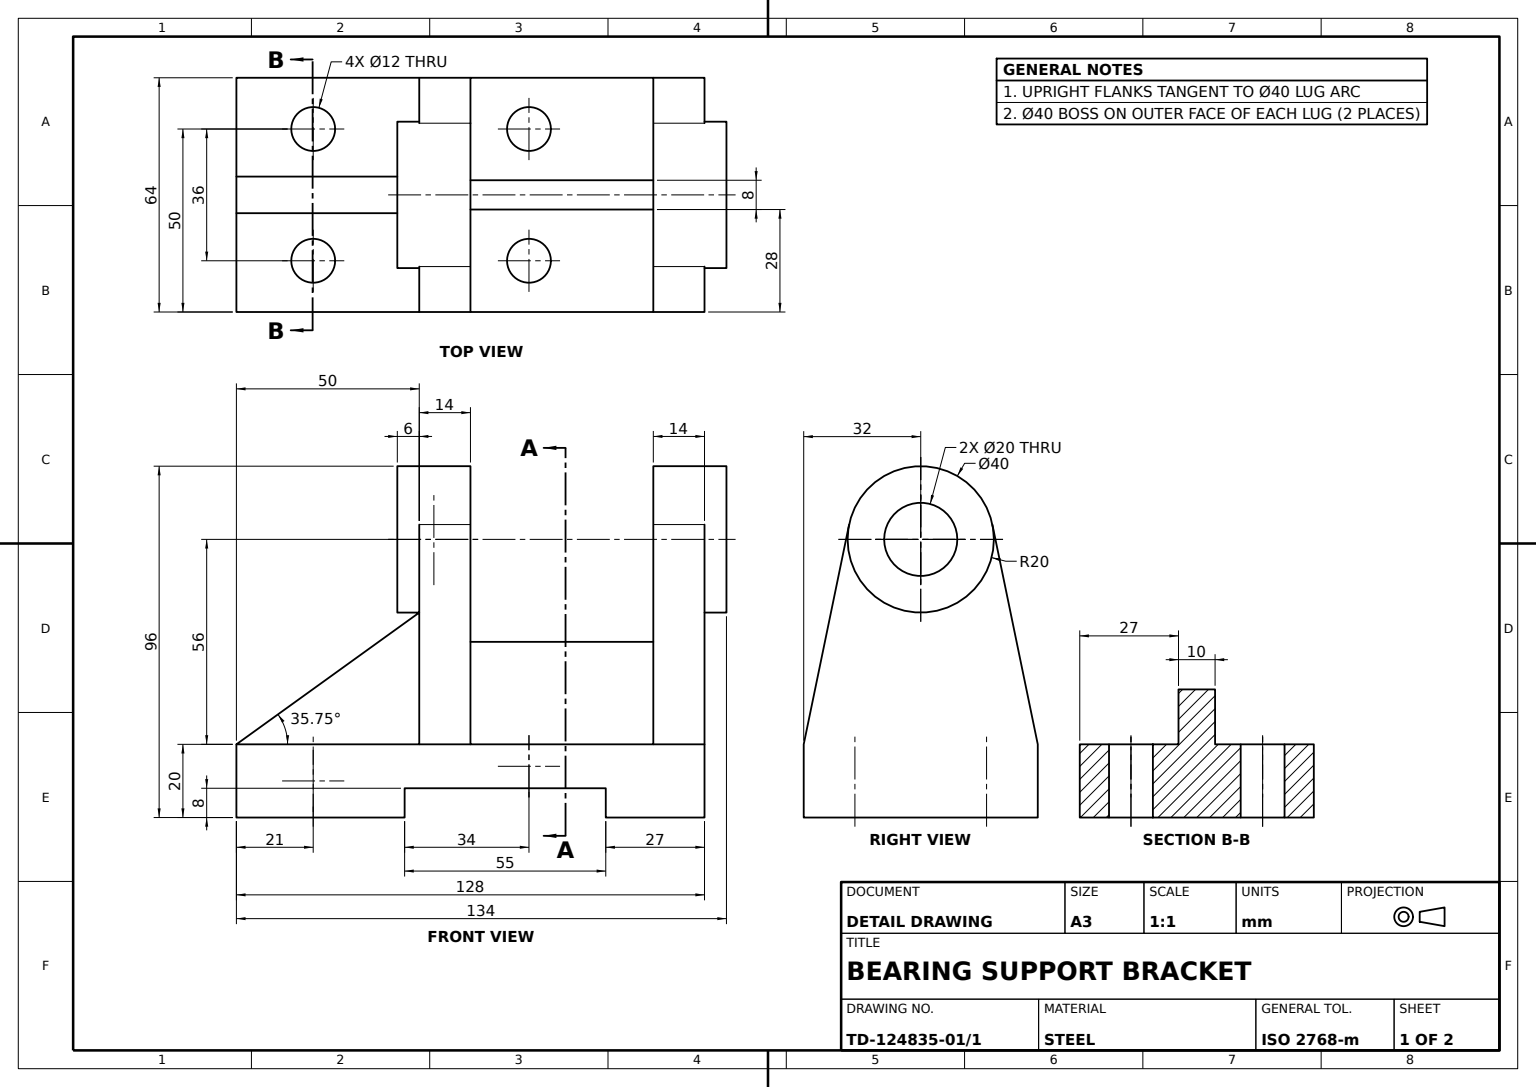
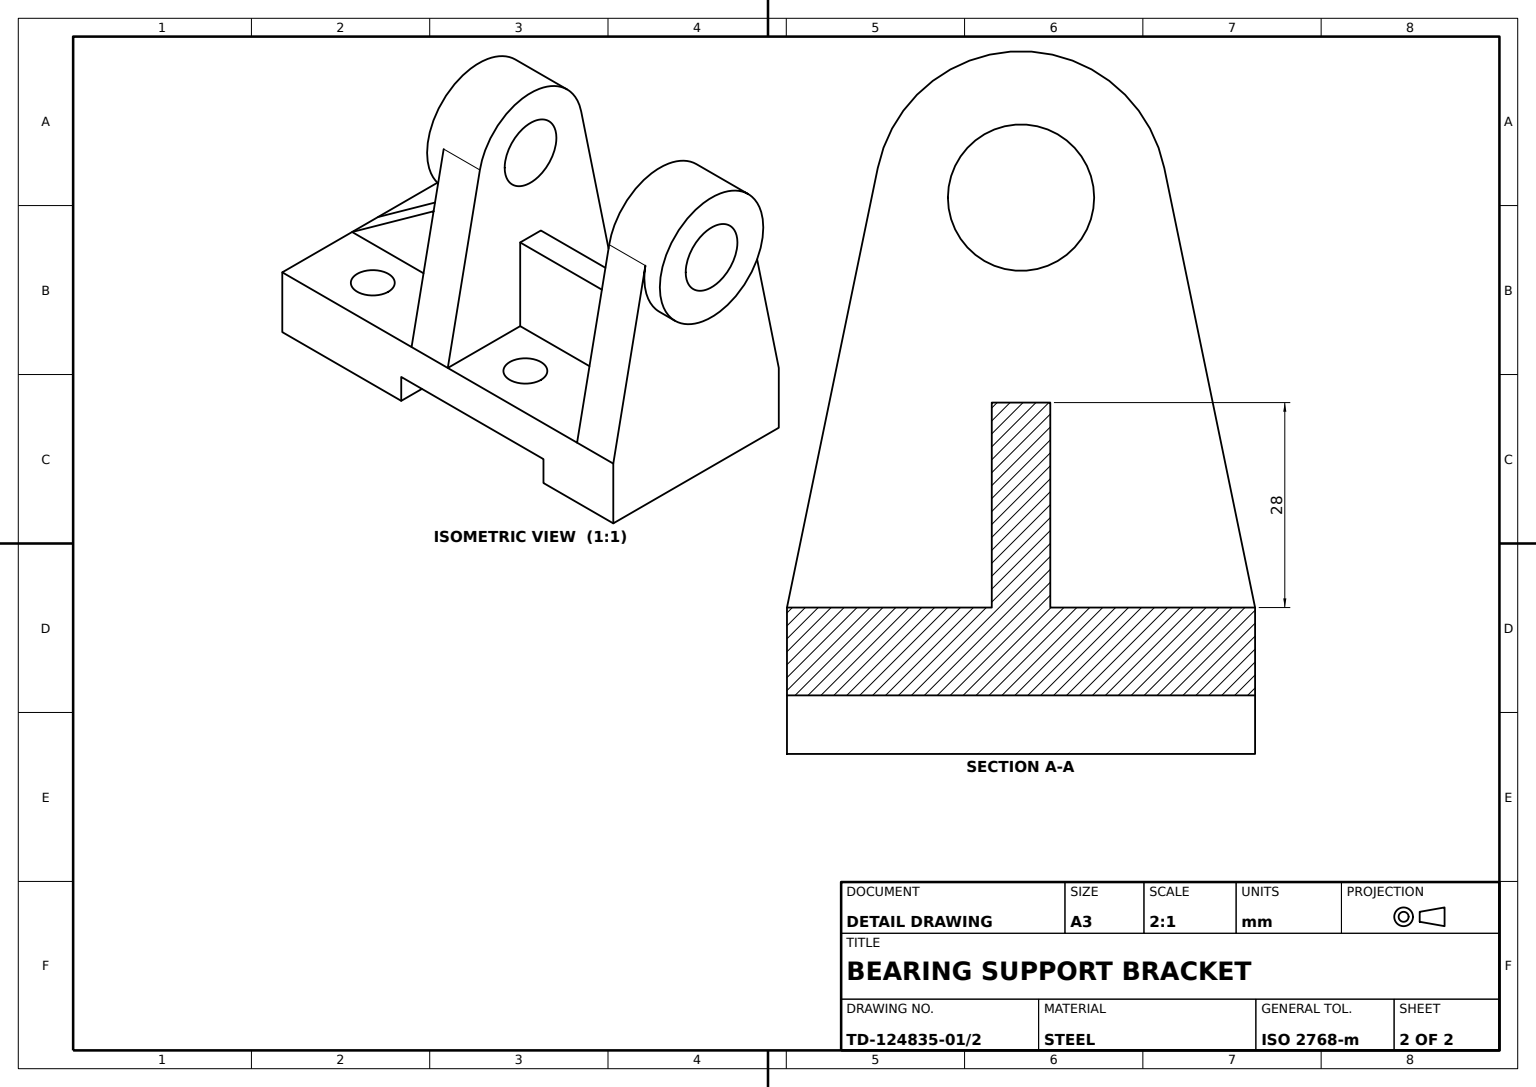
from build123d import *

# Parameters (mm, degrees)
BASE_PLATE_DEPTH           = 32
LUG_UPRIGHT_PROFILE_R      = 10
LUG_UPRIGHT_DEPTH          = 14
LUG_START                  = 6
SKETCH2_3_R                = 20
SKETCH2_3_R_2              = 10
LUG_HUB_BOSS_DEPTH         = 6
BACK_WEB_PROFILE_W         = 8
BACK_WEB_PROFILE_H         = 50
BACK_WEB_DEPTH             = 28
STIFFENING_RIB_REACH       = 165.169
STIFFENING_RIB_PATH_WALL_W = 389.948936072
STIFFENING_RIB_PATH_WALL_H = 10
MOUNTING_HOLES_PROFILE_R   = 6
MOUNTING_HOLES_DEPTH       = 153.262930485


with BuildPart() as part:
    # Base Plate Profile → Base Plate (new, symmetric)
    with BuildSketch(Plane(origin=(0, 0, 0), x_dir=(0, 0, -1), z_dir=(1, 0, 0))):
        Polygon((-82, 0), (-128, 0), (-128, 20), (0, 20), (0, 0), (-27, 0), (-27, 8), (-82, 8), align=None)
    extrude(amount=BASE_PLATE_DEPTH, both=True)

    # Lug Upright Profile → Lug Upright (add)
    with BuildSketch(Plane(origin=(0, 0, 0), x_dir=(-1, 0, 0), z_dir=(0, 0, -1))):
        with BuildLine():
            Line((-19.585841233, 80.049052133), (-32, 20))
            Line((-32, 20), (32, 20))
            Line((32, 20), (19.585841233, 80.049052133))
            ThreePointArc((19.585841233, 80.049052133), (0, 96), (-19.585841233, 80.049052133))
        make_face()
        with Locations((0, 76)):
            Circle(LUG_UPRIGHT_PROFILE_R, mode=Mode.SUBTRACT)
    lug_upright = extrude(amount=-LUG_UPRIGHT_DEPTH)

    # Sketch2_3 → Lug Hub Boss (add)
    with BuildSketch(Plane(origin=(0, 0, 0), x_dir=(-1, 0, 0), z_dir=(0, 0, -1)).offset(LUG_START)):
        with Locations((0, 76)):
            Circle(SKETCH2_3_R)
        with Locations((0, 76)):
            Circle(SKETCH2_3_R_2, mode=Mode.SUBTRACT)
    lug_hub_boss = extrude(amount=-LUG_HUB_BOSS_DEPTH)

    # Lug Mirror: Lug Upright, Lug Hub Boss across plane
    add(lug_upright.mirror(Plane.XY.offset(39)))
    add(lug_hub_boss.mirror(Plane.XY.offset(39)))

    # Back Web Profile → Back Web (add)
    with BuildSketch(Plane(origin=(0, 20, 0), x_dir=(1, 0, 0), z_dir=(0, 1, 0))):
        with Locations((0, -39)):
            Rectangle(BACK_WEB_PROFILE_W, BACK_WEB_PROFILE_H)
    extrude(amount=BACK_WEB_DEPTH)

    # Stiffening Rib Path wall → Stiffening Rib (add, up to next)
    with BuildSketch(Plane(origin=(0, 38, 103), x_dir=(0, 0.584304725845, -0.811534341451), z_dir=(0, 0.811534341451, 0.584304725845)), mode=Mode.PRIVATE) as stiffening_rib_sk1:
        Rectangle(STIFFENING_RIB_PATH_WALL_W, STIFFENING_RIB_PATH_WALL_H)
    stiffening_rib_tool1 = extrude(stiffening_rib_sk1.sketch, amount=-STIFFENING_RIB_REACH, mode=Mode.PRIVATE) - part.part
    add(stiffening_rib_tool1.solids().sort_by_distance((0, 38, 103))[0])

    # Mounting Holes Profile → Mounting Holes (cut, through all)
    with BuildSketch(Plane(origin=(0, 20, 0), x_dir=(1, 0, 0), z_dir=(0, 1, 0))):
        with Locations(Location((-18, -48, 0), (0, 0, 270))):
            Circle(MOUNTING_HOLES_PROFILE_R)
        with Locations(Location((18, -48, 0), (0, 0, 270))):
            Circle(MOUNTING_HOLES_PROFILE_R)
        with Locations(Location((18, -107, 0), (0, 0, 270))):
            Circle(MOUNTING_HOLES_PROFILE_R)
        with Locations(Location((-18, -107, 0), (0, 0, 270))):
            Circle(MOUNTING_HOLES_PROFILE_R)
    extrude(amount=-MOUNTING_HOLES_DEPTH, mode=Mode.SUBTRACT)


solid = part.part
